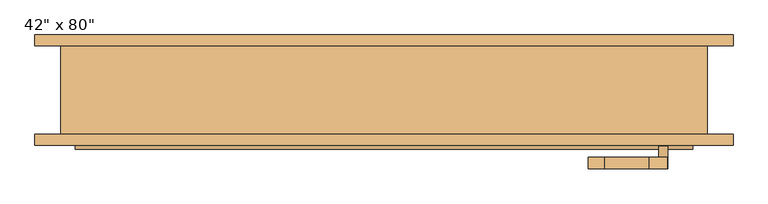
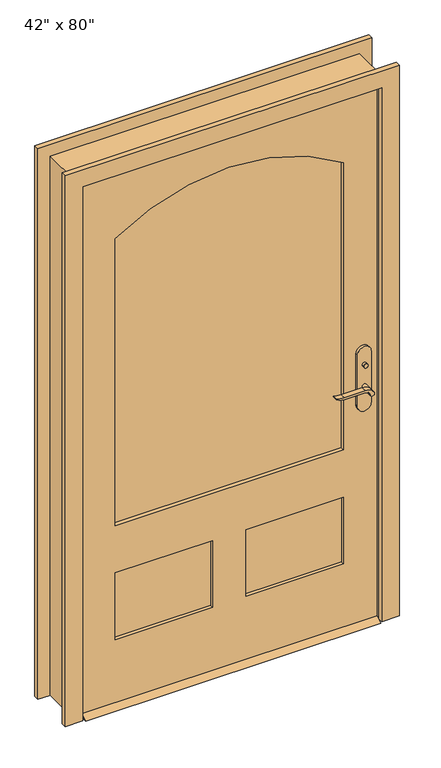
"""IFC4 building model written with IfcOpenShell, lengths in millimetres: door geometry."""

from ifc_helpers import new_model, si_unit, point, frame, frame_2d, origin, place, context, project, spatial, polyline, circle_curve, trimmed, segment, composite_curve, outline, extrude, faceted_brep, source, transform, mapped, element, save


def door_25c67de5(model_context):
    return source(origin(), model_context, "Body", "SolidModel", [
        extrude(outline(polyline([(-38.1, 12.7), (-12.7, 0.0), (-98.425, 0.0), (-73.025, 12.7), (-38.1, 12.7)])), frame((-533.4, 0.0, 0.0), z_axis=(1.0, 0.0, 0.0), x_axis=(0.0, 1.0, 0.0)), (0.0, 0.0, 1.0), 1066.8),
        extrude(outline(polyline([(487.6, -18.1), (487.6, -28.1), (477.6, -28.1), (477.6, -18.1), (487.6, -18.1)])), frame((0.0, 0.0, 981.9), z_axis=(0.0, 0.0, 1.0), x_axis=(1.0, 0.0, 0.0)), (0.0, 0.0, 1.0), 30.0),
        extrude(outline(composite_curve([segment(trimmed(circle_curve(frame_2d((996.9, 482.6)), 8.0), [point((996.9, 474.6))], [point((996.9, 490.6))], False, "CARTESIAN"), True, "CONTINUOUS"), segment(trimmed(circle_curve(frame_2d((996.9, 482.6)), 8.0), [point((996.9, 490.6))], [point((996.9, 474.6))], False, "CARTESIAN"), True, "CONTINUOUS")], self_intersect=False)), frame((0.0, -93.025, 0.0), z_axis=(0.0, 1.0, 0.0), x_axis=(0.0, 0.0, 1.0)), (0.0, 0.0, 1.0), 10.0),
        extrude(outline(composite_curve([segment(trimmed(circle_curve(frame_2d((897.1555521, 458.9324871)), 37.2832219), [point((919.0523287, 489.1081363))], [point((934.4, 457.2325667))], False, "CARTESIAN"), True, "CONTINUOUS"), segment(polyline([(934.4, 457.2325667), (934.4, 380.9564091)]), True, "CONTINUOUS"), segment(trimmed(circle_curve(frame_2d((1017.6850638, 381.0227909)), 83.2850902), [point((934.4, 380.9564091))], [point((939.4, 352.6))], True, "CARTESIAN"), True, "CONTINUOUS"), segment(polyline([(939.4, 352.6), (936.6135558, 352.6)]), True, "CONTINUOUS"), segment(trimmed(circle_curve(frame_2d((986.6709207, 384.5396612)), 59.3791355), [point((936.6135558, 352.6))], [point((927.4, 380.9564091))], False, "CARTESIAN"), True, "CONTINUOUS"), segment(polyline([(927.4, 380.9564091), (927.4, 457.2138099)]), True, "CONTINUOUS"), segment(trimmed(circle_curve(frame_2d((909.2738613, 457.2138099)), 18.1261387), [point((927.4, 457.2138099))], [point((914.4, 474.6))], True, "CARTESIAN"), True, "CONTINUOUS"), segment(trimmed(circle_curve(frame_2d((914.4, 482.6)), 8.0), [point((914.4, 474.6))], [point((919.0523287, 489.1081363))], False, "CARTESIAN"), True, "CONTINUOUS")], self_intersect=False)), frame((0.0, 1.9, 0.0), z_axis=(0.0, 1.0, 0.0), x_axis=(0.0, 0.0, 1.0)), (0.0, 0.0, 1.0), 20.0),
        extrude(outline(composite_curve([segment(trimmed(circle_curve(frame_2d((914.4, 482.6)), 8.0), [point((914.3999903, 474.6))], [point((919.0523287, 489.1081363))], False, "CARTESIAN"), True, "CONTINUOUS"), segment(trimmed(circle_curve(frame_2d((897.1555521, 458.9324871)), 37.2832219), [point((919.0523287, 489.1081363))], [point((934.4, 457.2325667))], False, "CARTESIAN"), True, "CONTINUOUS"), segment(polyline([(934.4, 457.2325667), (934.4, 380.9564091)]), True, "CONTINUOUS"), segment(trimmed(circle_curve(frame_2d((1017.6850638, 381.0227909)), 83.2850902), [point((934.4, 380.9564091))], [point((939.4, 352.6))], True, "CARTESIAN"), True, "CONTINUOUS"), segment(polyline([(939.4, 352.6), (936.6135558, 352.6)]), True, "CONTINUOUS"), segment(trimmed(circle_curve(frame_2d((986.6709207, 384.5396612)), 59.3791355), [point((936.6135558, 352.6))], [point((927.4, 380.9564091))], False, "CARTESIAN"), True, "CONTINUOUS"), segment(polyline([(927.4, 380.9564091), (927.4, 457.2138122)]), True, "CONTINUOUS"), segment(trimmed(circle_curve(frame_2d((909.2738682, 457.2138122)), 18.1261318), [point((927.4, 457.2138122))], [point((914.3999903, 474.6))], True, "CARTESIAN"), True, "CONTINUOUS")], self_intersect=False)), frame((0.0, -133.025, 0.0), z_axis=(0.0, 1.0, 0.0), x_axis=(0.0, 0.0, 1.0)), (0.0, 0.0, 1.0), 20.0),
        extrude(outline(composite_curve([segment(trimmed(circle_curve(frame_2d((914.4, 482.6)), 8.0), [point((914.4, 474.6))], [point((914.4, 490.6))], False, "CARTESIAN"), True, "CONTINUOUS"), segment(trimmed(circle_curve(frame_2d((914.4, 482.6)), 8.0), [point((914.4, 490.6))], [point((914.4, 474.6))], False, "CARTESIAN"), True, "CONTINUOUS")], self_intersect=False)), frame((0.0, -28.1, 0.0), z_axis=(0.0, 1.0, 0.0), x_axis=(0.0, 0.0, 1.0)), (0.0, 0.0, 1.0), 30.0),
        extrude(outline(composite_curve([segment(trimmed(circle_curve(frame_2d((914.4, 482.6)), 8.0), [point((914.4, 474.6))], [point((914.4, 490.6))], False, "CARTESIAN"), True, "CONTINUOUS"), segment(trimmed(circle_curve(frame_2d((914.4, 482.6)), 8.0), [point((914.4, 490.6))], [point((914.4, 474.6))], False, "CARTESIAN"), True, "CONTINUOUS")], self_intersect=False)), frame((0.0, -113.025, 0.0), z_axis=(0.0, 1.0, 0.0), x_axis=(0.0, 0.0, 1.0)), (0.0, 0.0, 1.0), 30.0),
        extrude(outline(composite_curve([segment(polyline([(844.4, 507.6), (1039.4, 507.6)]), True, "CONTINUOUS"), segment(trimmed(circle_curve(frame_2d((1039.4, 482.6)), 25.0), [point((1039.4, 507.6))], [point((1039.4, 457.6))], False, "CARTESIAN"), True, "CONTINUOUS"), segment(polyline([(1039.4, 457.6), (844.4, 457.6)]), True, "CONTINUOUS"), segment(trimmed(circle_curve(frame_2d((844.4, 482.6)), 25.0), [point((844.4, 457.6))], [point((844.4, 507.6))], False, "CARTESIAN"), True, "CONTINUOUS")], self_intersect=False)), frame((0.0, -38.1, 0.0), z_axis=(0.0, 1.0, 0.0), x_axis=(0.0, 0.0, 1.0)), (0.0, 0.0, 1.0), 10.0),
        extrude(outline(composite_curve([segment(polyline([(844.4, 507.6), (1039.4, 507.6)]), True, "CONTINUOUS"), segment(trimmed(circle_curve(frame_2d((1039.4, 482.6)), 25.0), [point((1039.4, 507.6))], [point((1039.4, 457.6))], False, "CARTESIAN"), True, "CONTINUOUS"), segment(polyline([(1039.4, 457.6), (844.4, 457.6)]), True, "CONTINUOUS"), segment(trimmed(circle_curve(frame_2d((844.4, 482.6)), 25.0), [point((844.4, 457.6))], [point((844.4, 507.6))], False, "CARTESIAN"), True, "CONTINUOUS")], self_intersect=False)), frame((0.0, -83.025, 0.0), z_axis=(0.0, 1.0, 0.0), x_axis=(0.0, 0.0, 1.0)), (0.0, 0.0, 1.0), 10.0),
        extrude(outline(polyline([(2032.0, -533.4), (12.7, -533.4), (12.7, 533.4), (2032.0, 533.4), (2032.0, -533.4)]), holes=[composite_curve([segment(polyline([(688.975, -412.75), (1784.35, -412.75)]), True, "CONTINUOUS"), segment(trimmed(circle_curve(frame_2d((1177.13125, 0.0)), 734.21875), [point((1784.35, -412.75))], [point((1784.35, 412.75))], True, "CARTESIAN"), True, "CONTINUOUS"), segment(polyline([(1784.35, 412.75), (688.975, 412.75), (688.975, -412.75)]), True, "CONTINUOUS")], self_intersect=False), polyline([(508.0, -60.325), (254.0, -60.325), (254.0, -412.75), (508.0, -412.75), (508.0, -60.325)]), polyline([(508.0, 412.75), (254.0, 412.75), (254.0, 60.325), (508.0, 60.325), (508.0, 412.75)])]), frame((0.0, -73.025, 0.0), z_axis=(0.0, 1.0, 0.0), x_axis=(0.0, 0.0, 1.0)), (0.0, 0.0, 1.0), 34.925),
        faceted_brep([(558.8, -73.025, 0.0), (533.4, -73.025, 0.0), (533.4, -38.1, 0.0), (520.7, -38.1, 0.0), (520.7, -3.175, 0.0), (533.4, -3.175, 0.0), (533.4, 79.375, 0.0), (558.8, 79.375, 0.0), (558.8, 79.375, 2057.4), (558.8, -73.025, 2057.4), (533.4, 79.375, 2032.0), (-533.4, 79.375, 2032.0), (-533.4, 79.375, 0.0), (-558.8, 79.375, 0.0), (-558.8, 79.375, 2057.4), (533.4, -3.175, 2032.0), (520.7, -3.175, 2019.3), (-520.7, -3.175, 2019.3), (-520.7, -3.175, 0.0), (-533.4, -3.175, 0.0), (-533.4, -3.175, 2032.0), (520.7, -38.1, 2019.3), (533.4, -38.1, 2032.0), (-533.4, -38.1, 2032.0), (-533.4, -38.1, 0.0), (-520.7, -38.1, 0.0), (-520.7, -38.1, 2019.3), (533.4, -73.025, 2032.0), (-558.8, -73.025, 2057.4), (-558.8, -73.025, 0.0), (-533.4, -73.025, 0.0), (-533.4, -73.025, 2032.0)], [[[0, 1, 2, 3, 4, 5, 6, 7]], [[7, 8, 9, 0]], [[6, 10, 11, 12, 13, 14, 8, 7]], [[5, 15, 10, 6]], [[4, 16, 17, 18, 19, 20, 15, 5]], [[3, 21, 16, 4]], [[2, 22, 23, 24, 25, 26, 21, 3]], [[1, 27, 22, 2]], [[0, 9, 28, 29, 30, 31, 27, 1]], [[8, 14, 28, 9]], [[15, 20, 11, 10]], [[21, 26, 17, 16]], [[27, 31, 23, 22]], [[29, 13, 12, 19, 18, 25, 24, 30]], [[14, 13, 29, 28]], [[20, 19, 12, 11]], [[26, 25, 18, 17]], [[31, 30, 24, 23]]]),
        extrude(outline(polyline([(-60.325, -49.7416667), (-60.325, -61.3833333), (-412.75, -61.3833333), (-412.75, -49.7416667), (-60.325, -49.7416667)])), frame((0.0, 0.0, 254.0), z_axis=(0.0, 0.0, 1.0), x_axis=(1.0, 0.0, 0.0)), (0.0, 0.0, 1.0), 254.0),
        extrude(outline(polyline([(412.75, -49.7416667), (412.75, -61.3833333), (60.325, -61.3833333), (60.325, -49.7416667), (412.75, -49.7416667)])), frame((0.0, 0.0, 254.0), z_axis=(0.0, 0.0, 1.0), x_axis=(1.0, 0.0, 0.0)), (0.0, 0.0, 1.0), 254.0),
        extrude(outline(composite_curve([segment(polyline([(688.975, -412.75), (688.975, 412.75), (1784.35, 412.75)]), True, "CONTINUOUS"), segment(trimmed(circle_curve(frame_2d((1177.13125, 0.0)), 734.21875), [point((1784.35, 412.75))], [point((1784.35, -412.75))], False, "CARTESIAN"), True, "CONTINUOUS"), segment(polyline([(1784.35, -412.75), (688.975, -412.75)]), True, "CONTINUOUS")], self_intersect=False)), frame((0.0, -59.055, 0.0), z_axis=(0.0, 1.0, 0.0), x_axis=(0.0, 0.0, 1.0)), (0.0, 0.0, 1.0), 6.985),
        extrude(outline(polyline([(0.0, -539.75), (2038.35, -539.75), (2038.35, 539.75), (0.0, 539.75), (0.0, 603.25), (2101.85, 603.25), (2101.85, -603.25), (0.0, -603.25), (0.0, -539.75)])), frame((0.0, 79.375, 0.0), z_axis=(0.0, 1.0, 0.0), x_axis=(0.0, 0.0, 1.0)), (0.0, 0.0, 1.0), 19.05),
        extrude(outline(polyline([(0.0, -539.75), (2038.35, -539.75), (2038.35, 539.75), (0.0, 539.75), (0.0, 603.25), (2101.85, 603.25), (2101.85, -603.25), (0.0, -603.25), (0.0, -539.75)])), frame((0.0, -92.075, 0.0), z_axis=(0.0, 1.0, 0.0), x_axis=(0.0, 0.0, 1.0)), (0.0, 0.0, 1.0), 19.05),
    ])


if __name__ == "__main__":
    model = new_model("IFC4")
    model_context = context("Model", 3, world=origin())
    ifc_project = project(units=[si_unit("LENGTHUNIT", "METRE", prefix="MILLI")], contexts=[model_context])
    site = spatial("IfcSite", under=ifc_project)
    building = spatial("IfcBuilding", under=site)
    placement = place(None, origin())
    door_shape = door_25c67de5(model_context)
    element("IfcDoor", 1, ObjectType="42\" x 80\"", at=placement, inside=building, context=model_context, shape_type="MappedRepresentation", body=[
        mapped(door_shape, transform((0.0, 0.0, 0.0), x_axis=(1.0, 0.0, 0.0), y_axis=(0.0, 1.0, 0.0), z_axis=(0.0, 0.0, 1.0))),
    ])
    save(model, "model.ifc")

# Revit data of these elements
# Type "42\" x 80\""
#   Type Mark = "9"
#   Assembly Code = "B2030100"
#   Analytic Construction = "French door, wood frame with single glass"
#   Threshold Offset [instance default] = 0' - 0 1/2"
#   Thickness = 0' - 1 3/8"
#   Thermal Resistance (R) = 1.0696 (h·ft²·°F)/BTU
#   Swing Angle [instance default] = 90.00°
#   Stiles = 0' - 4 3/4"
#   Rough Width = 3' - 8"
#   Rough Height = 6' - 9"
#   Radius = 2' - 4 29/32"
#   Lock Rail = 0' - 7 1/8"
#   Height = 6' - 8"
#   Width = 3' - 6"
#   Heat Transfer Coefficient (U) = 0.9350 BTU/(h·ft²·°F)
#   Door Offset [instance default] = 0' - 0"
#   Bottom Rail = 0' - 9 1/2"
#   Threshold [instance default] = yes
#   Function = 1
#   Exterior Trim [instance default] = yes
#   Trim Material = Cherry
#   Threshold Material = Cherry
#   Panel Material = Cherry
#   Glazing = Glass
#   Frame Material = Cherry
#   Door Handle Material = Aluminum
#   Visual Light Transmittance = 0
#   Solar Heat Gain Coefficient = 0
#   Wall Closure = (empty or 0)
#   Construction Type = (empty or 0)
# Element 1 (IfcDoor, "42\" x 80\"")
#   Materials on its faces: "Cherry", "Aluminum", "Glass"
# Materials
#   "Cherry": class "Wood", colour RGB 226 177 128, transparency 0, Description = "Prunus Serotina", Cost = 0
#   "Glass": class "Glass", colour RGB 0 128 192, transparency 0.75, Description = "Soda Lime Glass", Cost = 0
#   "Aluminum": class "Metal", colour RGB 247 247 247, transparency 0, Description = "Aluminum 6061", Cost = 0
